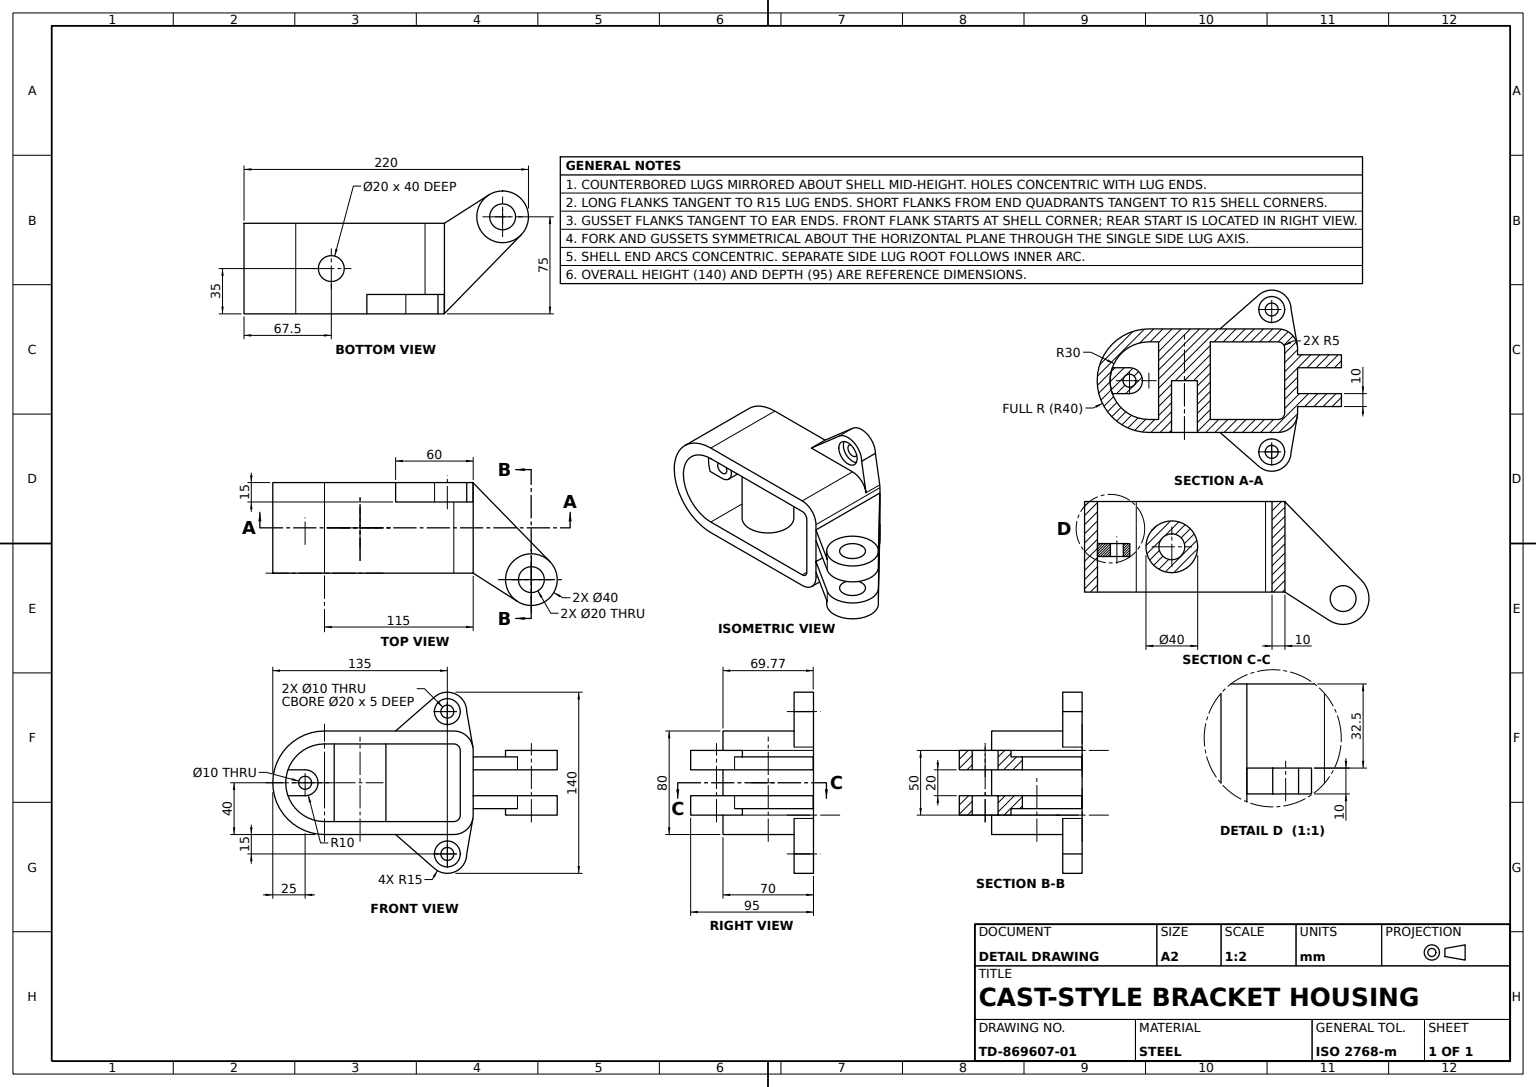
from build123d import *

# Parameters (mm, degrees)
HOUSING_SHELL_70MM_DEPTH      = 70
SKETCH1_3_R                   = 10
SKETCH1_3_R_2                 = 5
FRONT_LUG_BOSS_15MM_DEPTH     = 15
FRONT_START                   = 10
SKETCH1_6_R                   = 10
SKETCH1_6_R_2                 = 5
FRONT_LUG_CUT_5MM_DEPTH       = 5
SKETCH1_7_R                   = 5
FRONT_PROFILE_CUT_DEPTH       = 164.401346384
TOP_PROFILE_SKETCH_R          = 20
TOP_PROFILE_SKETCH_R_2        = 10
TOP_BOSS_PRIMARY_DEPTH        = 30
TOP_START                     = -30
SKETCH2_3_R                   = 20
SKETCH2_3_R_2                 = 10
TOP_BOSS_SECONDARY_DEPTH      = 30
TOP_START_2                   = -40
SKETCH2_4_R                   = 10
TOP_CUT_10MM_DEPTH            = 10
EAR_START                     = 10
EAR_BOSS_10MM_DEPTH           = 10
SKETCH4_3_R                   = 20
SKETCH4_3_R_2                 = 10
EAR_BOSS_15MM_DEPTH           = 15
SEPARATE_START                = 32.5
SKETCH1_8_R                   = 5
SEPARATE_BOSS_BODY_10MM_DEPTH = 10


with BuildPart() as part:
    # Front Profile Sketch → Housing Shell 70mm (new body)
    with BuildSketch(Plane.XY):
        with BuildLine():
            ThreePointArc((115, 40), (125.606601718, 35.606601718), (130, 25))
            Line((130, 25), (130, -25))
            ThreePointArc((130, -25), (125.606601718, -35.606601718), (115, -40))
            Line((115, -40), (15, -40))
            ThreePointArc((15, -40), (-25, 0), (15, 40))
            Line((15, 40), (115, 40))
        make_face()
        with BuildLine():
            ThreePointArc((15, 30), (-15, 0), (15, -30))
            Line((15, -30), (115, -30))
            ThreePointArc((115, -30), (118.535533906, -28.535533906), (120, -25))
            Line((120, -25), (120, 25))
            ThreePointArc((120, 25), (118.535533906, 28.535533906), (115, 30))
            Line((115, 30), (15, 30))
        make_face(mode=Mode.SUBTRACT)
    extrude(amount=HOUSING_SHELL_70MM_DEPTH)

    # Sketch1_3 → Front Lug Boss 15mm (add)
    # profile 1 of 6: a face of its own
    with BuildSketch(Plane.XY):
        with BuildLine():
            Line((100.136986301, 66.301369863), (70, 40))
            Line((70, 40), (115, 40))
            ThreePointArc((115, 40), (124.653687096, 36.480693597), (129.777469816, 27.574176728))
            Line((129.777469816, 27.574176728), (125, 55))
            ThreePointArc((125, 55), (116.207044165, 68.655497162), (100.136986301, 66.301369863))
        make_face()
        with Locations((110, 55)):
            Circle(SKETCH1_3_R, mode=Mode.SUBTRACT)
    # profile 2 of 6: a face of its own
    with BuildSketch(Plane.XY):
        with Locations((110, 55)):
            Circle(SKETCH1_3_R)
        with Locations((110, 55)):
            Circle(SKETCH1_3_R_2, mode=Mode.SUBTRACT)
    # profile 3 of 6: a face of its own
    with BuildSketch(Plane.XY):
        with Locations((110, 55)):
            Circle(SKETCH1_3_R_2)
    # profile 4 of 6: a face of its own
    with BuildSketch(Plane.XY):
        with BuildLine():
            Line((115, -40), (70, -40))
            Line((70, -40), (100.136986301, -66.301369863))
            ThreePointArc((100.136986301, -66.301369863), (116.207044165, -68.655497162), (125, -55))
            Line((125, -55), (129.777469816, -27.574176728))
            ThreePointArc((129.777469816, -27.574176728), (124.653687096, -36.480693597), (115, -40))
        make_face()
        with Locations((110, -55)):
            Circle(SKETCH1_3_R, mode=Mode.SUBTRACT)
    # profile 5 of 6: a face of its own
    with BuildSketch(Plane.XY):
        with Locations((110, -55)):
            Circle(SKETCH1_3_R)
        with Locations((110, -55)):
            Circle(SKETCH1_3_R_2, mode=Mode.SUBTRACT)
    # profile 6 of 6: a face of its own
    with BuildSketch(Plane.XY):
        with Locations((110, -55)):
            Circle(SKETCH1_3_R_2)
    extrude(amount=FRONT_LUG_BOSS_15MM_DEPTH)

    # Sketch1_6 → Front Lug Cut 5mm (cut)
    # profile 1 of 4: a face of its own
    with BuildSketch(Plane.XY.offset(FRONT_START)):
        with Locations((110, -55)):
            Circle(SKETCH1_6_R)
        with Locations((110, -55)):
            Circle(SKETCH1_6_R_2, mode=Mode.SUBTRACT)
    # profile 2 of 4: a face of its own
    with BuildSketch(Plane.XY.offset(FRONT_START)):
        with Locations((110, -55)):
            Circle(SKETCH1_6_R_2)
    # profile 3 of 4: a face of its own
    with BuildSketch(Plane.XY.offset(FRONT_START)):
        with Locations((110, 55)):
            Circle(SKETCH1_6_R)
        with Locations((110, 55)):
            Circle(SKETCH1_6_R_2, mode=Mode.SUBTRACT)
    # profile 4 of 4: a face of its own
    with BuildSketch(Plane.XY.offset(FRONT_START)):
        with Locations((110, 55)):
            Circle(SKETCH1_6_R_2)
    extrude(amount=FRONT_LUG_CUT_5MM_DEPTH, mode=Mode.SUBTRACT)

    # Sketch1_7 → Front Profile Cut (cut, through all)
    with BuildSketch(Plane.XY):
        with Locations((110, 55)):
            Circle(SKETCH1_7_R)
        with Locations((110, -55)):
            Circle(SKETCH1_7_R)
    extrude(amount=FRONT_PROFILE_CUT_DEPTH, mode=Mode.SUBTRACT)

    # Top Profile Sketch → Top Boss Primary (add)
    # profile 1 of 2: a face of its own
    with BuildSketch(Plane(origin=(0, 0, 0), x_dir=(1, 0, 0), z_dir=(0, 1, 0))):
        with Locations(Location((42.5, -35, 0), (0, 0, 270))):
            Circle(TOP_PROFILE_SKETCH_R)
        with Locations((42.5, -35)):
            Circle(TOP_PROFILE_SKETCH_R_2, mode=Mode.SUBTRACT)
    # profile 2 of 2: a face of its own
    with BuildSketch(Plane(origin=(0, 0, 0), x_dir=(1, 0, 0), z_dir=(0, 1, 0))):
        with Locations((42.5, -35)):
            Circle(TOP_PROFILE_SKETCH_R_2)
    extrude(amount=TOP_BOSS_PRIMARY_DEPTH)

    # Sketch2_3 → Top Boss Secondary (add)
    with BuildSketch(Plane(origin=(0, 0, 0), x_dir=(1, 0, 0), z_dir=(0, 1, 0)).offset(TOP_START)):
        with Locations(Location((42.5, -35, 0), (0, 0, 90))):
            Circle(SKETCH2_3_R)
        with Locations(Location((42.5, -35, 0), (0, 0, 270))):
            Circle(SKETCH2_3_R_2, mode=Mode.SUBTRACT)
    extrude(amount=TOP_BOSS_SECONDARY_DEPTH)

    # Sketch2_4 → Top Cut 10mm (cut)
    with BuildSketch(Plane(origin=(0, 0, 0), x_dir=(1, 0, 0), z_dir=(0, 1, 0)).offset(TOP_START_2)):
        with Locations(Location((42.5, -35, 0), (0, 0, 270))):
            Circle(SKETCH2_4_R)
    extrude(amount=TOP_CUT_10MM_DEPTH, mode=Mode.SUBTRACT)

    # Ear Profile Sketch → Ear Boss 10mm (add)
    with BuildSketch(Plane(origin=(0, 0, 0), x_dir=(1, 0, 0), z_dir=(0, 1, 0)).offset(EAR_START)):
        with BuildLine():
            Line((130, -70), (164.238039414, -91.857645278))
            ThreePointArc((164.238039414, -91.857645278), (159.486208673, -62.377707075), (189.316428168, -61.034331934))
            Line((189.316428168, -61.034331934), (129.777469816, 0))
            Line((129.777469816, 0), (130, -70))
        make_face()
    ear_boss_10mm = extrude(amount=EAR_BOSS_10MM_DEPTH)

    # Sketch4_3 → Ear Boss 15mm (add)
    with BuildSketch(Plane(origin=(0, 0, 0), x_dir=(1, 0, 0), z_dir=(0, 1, 0)).offset(EAR_START)):
        with Locations(Location((175, -75, 0), (0, 0, 44.28944294))):
            Circle(SKETCH4_3_R)
        with Locations(Location((175, -75, 0), (0, 0, 270))):
            Circle(SKETCH4_3_R_2, mode=Mode.SUBTRACT)
    ear_boss_15mm = extrude(amount=EAR_BOSS_15MM_DEPTH)

    # Ear Bosses Mirror: Ear Boss 10mm, Ear Boss 15mm across plane
    add(ear_boss_10mm.mirror(Plane.ZX))
    add(ear_boss_15mm.mirror(Plane.ZX))


with BuildPart() as body_2:
    # Sketch1_8 → Separate Boss Body 10mm (new body)
    with BuildSketch(Plane.XY.offset(SEPARATE_START)):
        with BuildLine():
            Line((0, 10), (-13.284271247, 10))
            ThreePointArc((-13.284271247, 10), (-15, 0), (-13.284271247, -10))
            Line((-13.284271247, -10), (0, -10))
            ThreePointArc((0, -10), (10, 0), (0, 10))
        make_face()
        Circle(SKETCH1_8_R, mode=Mode.SUBTRACT)
    extrude(amount=SEPARATE_BOSS_BODY_10MM_DEPTH)


solid = Compound([part.part, body_2.part])
